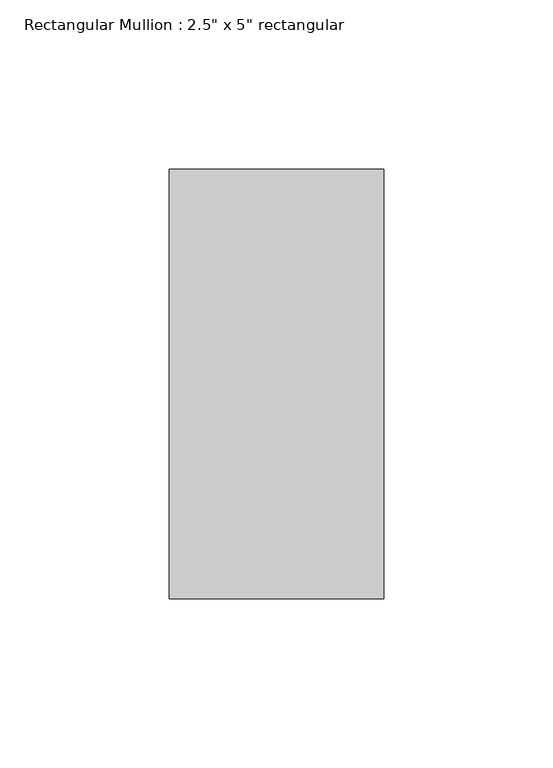
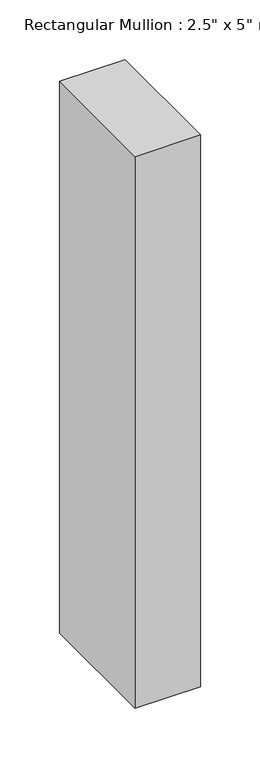
"""IFC4 building model written with IfcOpenShell, lengths in millimetres: member geometry."""

from ifc_helpers import new_model, si_unit, frame, origin, place, context, project, spatial, polyline, outline, extrude, source, transform, mapped, element, save


def member_6f432376(model_context):
    return source(origin(), model_context, "Body", "SweptSolid", [
        extrude(outline(polyline([(0.0, 63.5), (0.0, -63.5), (-63.5, -63.5), (-63.5, 63.5), (0.0, 63.5)])), frame((0.0, 0.0, -565.15), z_axis=(0.0, 0.0, 1.0), x_axis=(1.0, 0.0, 0.0)), (0.0, 0.0, 1.0), 565.15),
    ])


if __name__ == "__main__":
    model = new_model("IFC4")
    model_context = context("Model", 3, world=origin())
    ifc_project = project(units=[si_unit("LENGTHUNIT", "METRE", prefix="MILLI")], contexts=[model_context])
    site = spatial("IfcSite", under=ifc_project)
    building = spatial("IfcBuilding", under=site)
    placement = place(None, origin())
    member_shape = member_6f432376(model_context)
    element("IfcMember", 1, ObjectType="Rectangular Mullion : 2.5\" x 5\" rectangular", at=placement, inside=building, context=model_context, shape_type="MappedRepresentation", body=[
        mapped(member_shape, transform((0.0, 0.0, 0.0), x_axis=(1.0, 0.0, 0.0), y_axis=(0.0, 1.0, 0.0), z_axis=(0.0, 0.0, 1.0))),
    ])
    save(model, "model.ifc")

# Revit data of these elements
# Type "Rectangular Mullion : 2.5\" x 5\" rectangular"
#   built-in parameter 1007304 = 0.416667 (stored number, unit not read)
#   built-in parameter 1007301 = 0.104167 (stored number, unit not read)
#   built-in parameter 1007300 = 0.104167 (stored number, unit not read)
